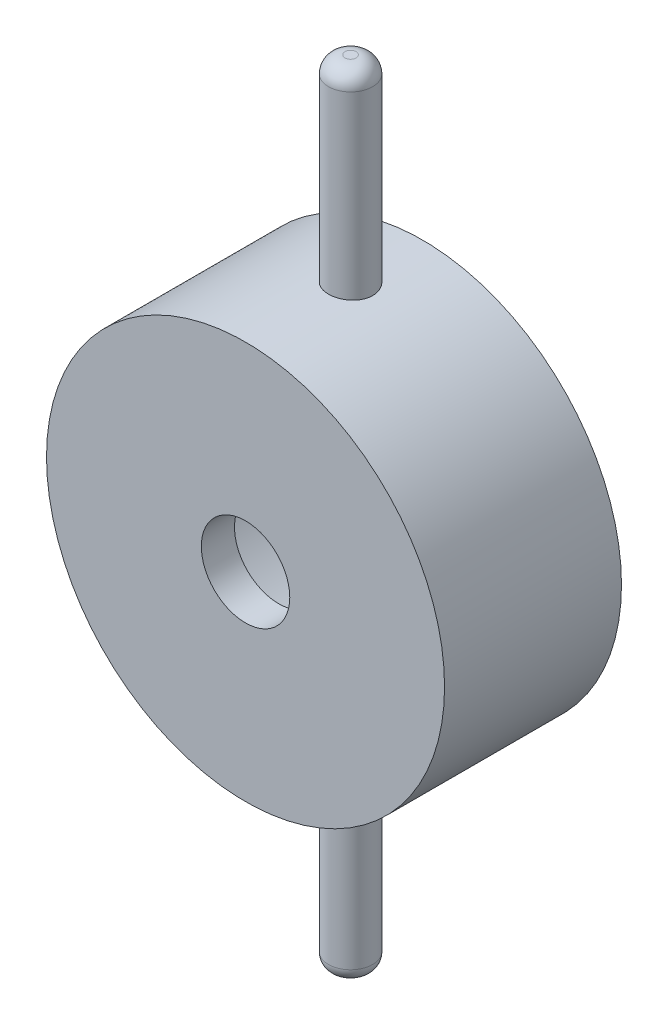
from build123d import *

# Parameters (mm, degrees)
HUB_PROFILE_SKETCH_R       = 36
HUB_72X32_DEPTH            = 32
HANDLE_START               = 35.5
HANDLE_PIN_SKETCH_8_R      = 4
HANDLE_PIN_8_DEPTH         = 36
PIN_END_FILLET_R3_R        = 3
FACE_RECESS_SKETCH_16_R    = 8
FACE_RECESS_16X6_DEPTH     = 6
MIRRORED_PIN_FILLET_R2_5_R = 2.5


with BuildPart() as part:
    # Hub Profile Sketch → Hub Ø72x32 (new body)
    with BuildSketch(Plane.XY):
        Circle(HUB_PROFILE_SKETCH_R)
    extrude(amount=HUB_72X32_DEPTH)

    # Handle Pin Sketch Ø8 → Handle Pin Ø8 (add)
    with BuildSketch(Plane(origin=(0, 0, 0), x_dir=(1, 0, 0), z_dir=(0, 1, 0)).offset(HANDLE_START)):
        with Locations(Location((0, -13, 0), (0, 0, 90))):
            Circle(HANDLE_PIN_SKETCH_8_R)
    handle_pin_8 = extrude(amount=HANDLE_PIN_8_DEPTH)

    # Pin End Fillet R3
    pin_end_fillet_r3_edges = [part.edges().sort_by_distance(p)[0] for p in [
        (0, 71.5, 17),
    ]]
    fillet(pin_end_fillet_r3_edges, radius=PIN_END_FILLET_R3_R)

    # Handle Pin Mirror: Handle Pin Ø8 across plane
    add(handle_pin_8.mirror(Plane.ZX))

    # Revolved Cut Sketch → Revolved Cut (revolve, cut)
    with BuildSketch(Plane(origin=(0, 0, 0), x_dir=(1, 0, 0), z_dir=(0, 1, 0))):
        Polygon((0, -26), (-10, -26), (-10, -28), (-28, -28), (-28, 0), (0, 0), align=None)
    revolve(axis=Axis((0, 0, -9.53547678), (0, 0, 1)), mode=Mode.SUBTRACT)

    # Face Recess Sketch Ø16 → Face Recess Ø16x6 (cut)
    with BuildSketch(Plane.XY.offset(32)):
        Circle(FACE_RECESS_SKETCH_16_R)
    extrude(amount=-FACE_RECESS_16X6_DEPTH, mode=Mode.SUBTRACT)

    # Mirrored Pin Fillet R2.5
    mirrored_pin_fillet_r2_5_edges = [part.edges().sort_by_distance(p)[0] for p in [
        (0, -71.5, 17),
    ]]
    fillet(mirrored_pin_fillet_r2_5_edges, radius=MIRRORED_PIN_FILLET_R2_5_R)


solid = part.part
